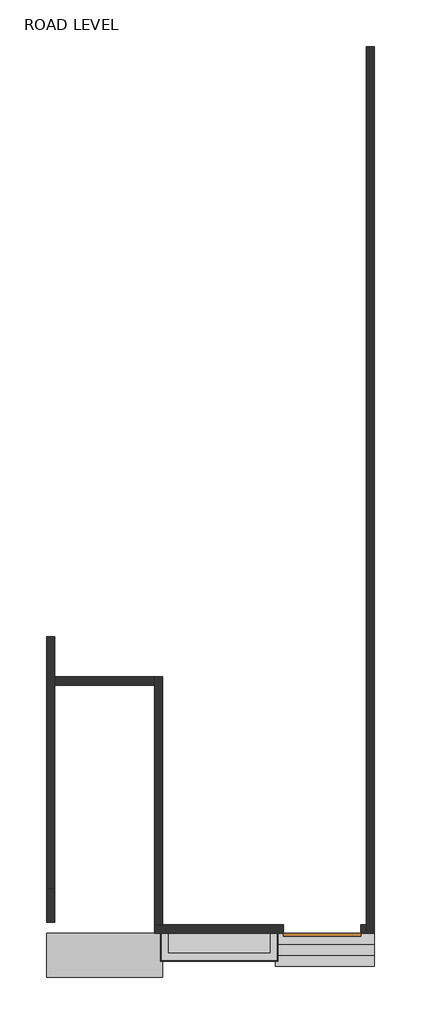
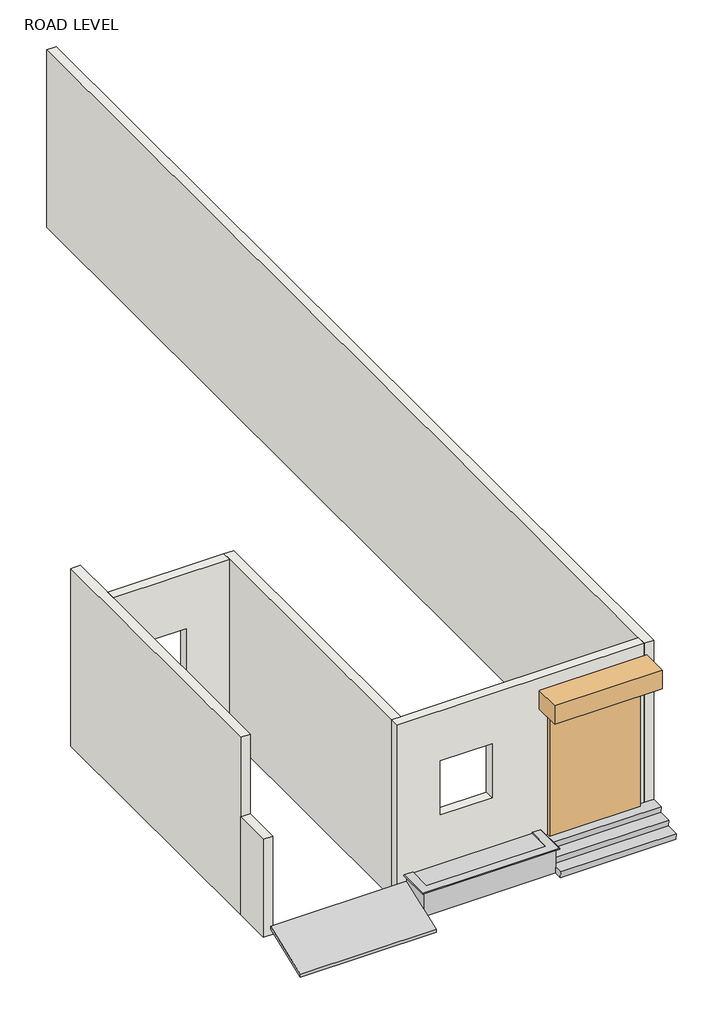
# One storey: 6 walls, 1 door, 1 proxy, 1 ramp, 1 stair flight.
"""IFC4 building model written with IfcOpenShell, lengths in millimetres."""

from ifc_helpers import new_model, si_unit, frame, origin, origin_with_axes, place, context, project, spatial, polyline, outline, extrude, faceted_brep, transform, mapped, element, save
from components import generic_models_2_generic_models_2_8e2cd793, m_door_overhead_rolling_2134_x_3658mm_be0fe279, ramp_3_52017588

model = new_model("IFC4")

# Units and contexts
model_context = context("Model", 3, world=origin())
ifc_project = project(units=[si_unit("LENGTHUNIT", "METRE", prefix="MILLI")], contexts=[model_context])

# Site, building, storey
site = spatial("IfcSite", under=ifc_project)
building = spatial("IfcBuilding", under=site)
storey = spatial("IfcBuildingStorey", under=building, Name="ROAD LEVEL", Elevation=0.0)

# Proxy
placement = place(None, origin())
generic_models_2_generic_models_2_shape = generic_models_2_generic_models_2_8e2cd793(model_context)
element("IfcBuildingElementProxy", 1, Name="Generic Models 2 : Generic Models 2", ObjectType="Generic Models 2 : Generic Models 2", at=placement, inside=storey, context=model_context, shape_type="MappedRepresentation", body=[
    mapped(generic_models_2_generic_models_2_shape, transform((0.0, 0.0, 0.0), x_axis=(1.0, 0.0, 0.0), y_axis=(0.0, 1.0, 0.0), z_axis=(0.0, 0.0, 1.0))),
])

# Door
m_door_overhead_rolling_2134_x_3658mm_shape = m_door_overhead_rolling_2134_x_3658mm_be0fe279(model_context)
element("IfcDoor", 2, ObjectType="M_Door-Overhead-Rolling : 2134 x 3658mm", at=placement, inside=storey, context=model_context, shape_type="MappedRepresentation", body=[
    mapped(m_door_overhead_rolling_2134_x_3658mm_shape, transform((7741.7271331, -11861.4643494, 0.0), x_axis=(1.0, 0.0, 0.0), y_axis=(0.0, 1.0, 0.0), z_axis=(0.0, 0.0, 1.0))),
])

# Ramp
ramp_3_shape = ramp_3_52017588(model_context)
element("IfcRamp", 3, ObjectType="Ramp 3", at=placement, inside=storey, context=model_context, shape_type="MappedRepresentation", body=[
    mapped(ramp_3_shape, transform((0.0, 0.0, 0.0), x_axis=(1.0, 0.0, 0.0), y_axis=(0.0, 1.0, 0.0), z_axis=(0.0, 0.0, 1.0))),
])

# Stair flight
element("IfcStairFlight", 4, ObjectType="3/4\" Nosing", at=placement, inside=storey, context=model_context, shape_type="Brep", body=[
    faceted_brep([(9176.8271331, -12890.1643494, 152.4), (6457.7191987, -12890.1643494, 152.4), (6457.7191987, -12871.1143494, 0.0), (9176.8271331, -12871.1143494, 0.0), (9176.8271331, -12566.3143494, 152.4), (6457.7191987, -12566.3143494, 152.4), (6457.7191987, -12566.3143494, 81.4048417), (6457.7191987, -12729.1240329, 0.0), (9176.8271331, -12729.1240329, 0.0), (9176.8271331, -12566.3143494, 81.4048417), (6457.7191987, -12585.3643494, 304.8), (9176.8271331, -12585.3643494, 304.8), (9176.8271331, -12261.5143494, 304.8), (6457.7191987, -12261.5143494, 304.8), (6457.7191987, -12261.5143494, 233.8048417), (9176.8271331, -12261.5143494, 233.8048417), (6457.7191987, -12280.5643494, 457.2), (9176.8271331, -12280.5643494, 457.2), (9176.8271331, -11975.7643494, 457.2), (6457.7191987, -11975.7643494, 457.2), (6457.7191987, -11975.7643494, 376.6798417), (9176.8271331, -11975.7643494, 376.6798417)], [[[0, 1, 2, 3]], [[1, 0, 4, 5]], [[1, 5, 6, 7, 2]], [[4, 0, 3, 8, 9]], [[10, 11, 12, 13]], [[10, 13, 14, 6, 5]], [[12, 11, 4, 9, 15]], [[5, 4, 11, 10]], [[16, 17, 18, 19]], [[16, 19, 20, 14, 13]], [[18, 17, 12, 15, 21]], [[19, 18, 21, 20]], [[13, 12, 17, 16]], [[3, 2, 7, 8]], [[8, 7, 6, 14, 20, 21, 15, 9]]]),
])

# Walls
element("IfcWall", 5, ObjectType="9\"", at=placement, inside=storey, context=model_context, shape_type="Brep", body=[
    faceted_brep([(8948.2271331, 12408.2356506, 0.0), (8948.2271331, -11747.1643494, 0.0), (8948.2271331, -11975.7643494, 0.0), (8948.2271331, -11975.7643494, 4419.6), (8948.2271331, -11747.1643494, 4419.6), (8948.2271331, 12408.2356506, 4419.6), (9176.8271331, 12408.2356506, 0.0), (9176.8271331, 12408.2356506, 4419.6), (9176.8271331, -11975.7643494, 4419.6), (9176.8271331, -11975.7643494, 0.0)], [[[0, 1, 2, 3, 4, 5]], [[6, 7, 8, 9]], [[2, 1, 0, 6, 9]], [[5, 4, 3, 8, 7]], [[0, 5, 7, 6]], [[3, 2, 9, 8]]]),
])
element("IfcWall", 6, ObjectType="9\"", at=placement, inside=storey, context=model_context, shape_type="Brep", body=[
    faceted_brep([(3118.9271331, -11747.1643494, 4419.6), (3347.5271331, -11747.1643494, 4419.6), (8948.2271331, -11747.1643494, 4419.6), (8948.2271331, -11747.1643494, 0.0), (8808.5271331, -11747.1643494, 0.0), (8808.5271331, -11747.1643494, 3657.6), (6674.9271331, -11747.1643494, 3657.6), (6674.9271331, -11747.1643494, 0.0), (3347.5271331, -11747.1643494, 0.0), (3118.9271331, -11747.1643494, 0.0), (4147.6271331, -11747.1643494, 3175.0), (4147.6271331, -11747.1643494, 1828.8), (5366.8271331, -11747.1643494, 1828.8), (5366.8271331, -11747.1643494, 3175.0), (8948.2271331, -11975.7643494, 4419.6), (3118.9271331, -11975.7643494, 4419.6), (3118.9271331, -11975.7643494, 0.0), (6674.9271331, -11975.7643494, 0.0), (6674.9271331, -11975.7643494, 3657.6), (8808.5271331, -11975.7643494, 3657.6), (8808.5271331, -11975.7643494, 0.0), (8948.2271331, -11975.7643494, 0.0), (4147.6271331, -11975.7643494, 3175.0), (5366.8271331, -11975.7643494, 3175.0), (5366.8271331, -11975.7643494, 1828.8), (4147.6271331, -11975.7643494, 1828.8)], [[[0, 1, 2, 3, 4, 5, 6, 7, 8, 9], [10, 11, 12, 13]], [[14, 15, 16, 17, 18, 19, 20, 21], [22, 23, 24, 25]], [[3, 21, 20, 4]], [[16, 9, 8, 7, 17]], [[2, 1, 0, 15, 14]], [[3, 2, 14, 21]], [[0, 9, 16, 15]], [[19, 5, 4, 20]], [[5, 19, 18, 6]], [[6, 18, 17, 7]], [[11, 10, 22, 25]], [[12, 11, 25, 24]], [[13, 12, 24, 23]], [[10, 13, 23, 22]]]),
])
element("IfcWall", 7, ObjectType="9\"", at=placement, inside=storey, context=model_context, shape_type="Brep", body=[
    faceted_brep([(3347.5271331, -11747.1643494, 0.0), (3347.5271331, -4927.2643494, 0.0), (3347.5271331, -4927.2643494, 4419.6), (3347.5271331, -11747.1643494, 4419.6), (3118.9271331, -11747.1643494, 0.0), (3118.9271331, -11747.1643494, 4419.6), (3118.9271331, -5155.8643494, 4419.6), (3118.9271331, -4927.2643494, 4419.6), (3118.9271331, -4927.2643494, 0.0), (3118.9271331, -5155.8643494, 0.0)], [[[0, 1, 2, 3]], [[4, 5, 6, 7, 8, 9]], [[1, 0, 4, 9, 8]], [[3, 2, 7, 6, 5]], [[0, 3, 5, 4]], [[2, 1, 8, 7]]]),
])
element("IfcWall", 8, ObjectType="9\"", at=placement, inside=storey, context=model_context, shape_type="SweptSolid", body=[
    extrude(outline(polyline([(0.0, 3118.9271331), (4419.6, 3118.9271331), (4419.6, 375.7271331), (0.0, 375.7271331), (0.0, 3118.9271331)]), holes=[polyline([(3048.0, 553.5271331), (3048.0, 2102.9271331), (1828.8, 2102.9271331), (1828.8, 553.5271331), (3048.0, 553.5271331)])]), frame((0.0, -5155.8643494, 0.0), z_axis=(0.0, 1.0, 0.0), x_axis=(0.0, 0.0, 1.0)), (0.0, 0.0, 1.0), 228.6),
])
element("IfcWall", 9, ObjectType="9\"", at=placement, inside=storey, context=model_context, shape_type="Brep", body=[
    faceted_brep([(147.1271331, -3822.3643494, 0.0), (147.1271331, -10756.5643494, 0.0), (147.1271331, -10756.5643494, 2438.4), (147.1271331, -10756.5643494, 4419.6), (147.1271331, -3822.3643494, 4419.6), (375.7271331, -3822.3643494, 0.0), (375.7271331, -3822.3643494, 4419.6), (375.7271331, -4927.2643494, 4419.6), (375.7271331, -5155.8643494, 4419.6), (375.7271331, -10756.5643494, 4419.6), (375.7271331, -10756.5643494, 2438.4), (375.7271331, -10756.5643494, 0.0), (375.7271331, -5155.8643494, 0.0), (375.7271331, -4927.2643494, 0.0)], [[[0, 1, 2, 3, 4]], [[5, 6, 7, 8, 9, 10, 11, 12, 13]], [[1, 0, 5, 13, 12, 11]], [[3, 2, 1, 11, 10, 9]], [[4, 3, 9, 8, 7, 6]], [[0, 4, 6, 5]]]),
])
element("IfcWall", 10, ObjectType="9\"", at=placement, inside=storey, context=model_context, shape_type="SweptSolid", body=[
    extrude(outline(polyline([(147.1271331, -11677.9324242), (147.1271331, -10756.5643494), (375.7271331, -10756.5643494), (375.7271331, -11677.9324242), (147.1271331, -11677.9324242)])), origin_with_axes(), (0.0, 0.0, 1.0), 2438.4),
])

save(model, "model.ifc")

# Revit data of these elements
# Type "M_Door-Overhead-Rolling : 2134 x 3658mm"
#   Type Mark = "8"
#   Construction Type Id = "MDOOR"
#   Assembly Code = "B2030400"
#   Analytic Construction = "Metal"
#   Thickness = 0' - 3.14961"
#   Rough Width [instance default] = 13' - 9.35433"
#   Rough Height [instance default] = 13' - 9.35433"
#   Heat Transfer Coefficient (U) = 0.651978 BTU/(h·ft²·°F)
#   Height [instance default] = 13' - 9.35433"
#   Width [instance default] = 13' - 9.35433"
#   Define Thermal Properties by = 1
#   Function = 1
#   Roller Material = Steel, Paint Finish, Ivory, Matte
#   Roller Box Material = Steel, Paint Finish, Ivory, Matte
#   Visual Light Transmittance = 0
#   Solar Heat Gain Coefficient = 0
#   Wall Closure = (empty or 0)
# Type "Ramp 3"
#   Assembly Code = "B1010600"
#   built-in parameter 1008304 = 0.25 (stored number, unit not read)
#   built-in parameter 1008303 = 30 (stored number, unit not read)
#   built-in parameter 1008301 = 2.66 (stored number, unit not read)
#   Function = 0
#   built-in parameter 1008308 = ramp
# Type "9\""
#   Assembly Code = "B2010"
#   Layers, outside or top first: 0' - 9" no material (function 1)
# Element 1 (IfcBuildingElementProxy, "Generic Models 2 : Generic Models 2")
#   Phase Created = New Construction
#   Materials on its faces: "Roofing, EPDM Membrane", "Oak Flooring", "Tile, Mosaic, Gray"
# Element 2 (IfcDoor, "M_Door-Overhead-Rolling : 2134 x 3658mm")
#   Width = 7' - 0"
#   Rough Width = 7' - 0"
#   Rough Height = 12' - 0"
#   Height = 12' - 0"
#   Phase Created = New Construction
#   Materials on its faces: "Steel, Paint Finish, Ivory, Matte"
# Element 3 (IfcRamp, "Ramp 3")
#   built-in parameter 1007275 = "DN"
#   built-in parameter 1007272 = "UP"
#   Width = 3' - 0"
#   built-in parameter 1007276 = 1
#   built-in parameter 1007274 = 1
#   built-in parameter 1007273 = 1
#   built-in parameter 1007271 = 1
#   Phase Created = New Construction
#   Materials on its faces: "ramp"
# Element 4 (IfcStairFlight, "3/4\" Nosing")
#   Phase Created = New Construction
#   Materials on its faces: "Gypsum Wall Board"
# Elements 5, 6, 7, 8, 9 (IfcWall, "9\"")
#   Top Offset = 0' - 0"
#   Base Offset = 0' - 0"
#   wall height = 14' - 6"
#   Phase Created = New Construction
#   Base Constraint = ROAD LEVEL
#   Top Constraint = FIRST FLOOR LEVEL
#   Materials on its faces: "Default Wall"
# Element 10 (IfcWall, "9\"")
#   Top Offset = 0' - 0"
#   Base Offset = 0' - 0"
#   Unconnected Height = 8' - 0"
#   wall height = 8' - 0"
#   Phase Created = New Construction
#   Base Constraint = ROAD LEVEL
#   Materials on its faces: "Default Wall"
# Materials
#   "Steel, Paint Finish, Ivory, Matte": class "Metal", colour RGB 247 247 239, transparency 0, Description = "Steel, paint finish, ivory, matte", Cost = 0
#   "ramp": class "Generic", colour RGB 123 104 76, transparency 0, Cost = 0
#   "Roofing, EPDM Membrane": class "Generic", colour RGB 127 127 127, transparency 0, Description = "EPDM roof membrane", Cost = 0
#   "Oak Flooring": class "Wood", colour RGB 216 169 114, transparency 0, Description = "Quercus Rubra", Cost = 0
#   "Tile, Mosaic, Gray": class "Generic", colour RGB 127 127 127, transparency 0, Description = "Mosiac tile, gray", Cost = 0
#   "Gypsum Wall Board": class "Generic", colour RGB 228 228 228, transparency 0, Description = "Gypsum Wall Board", Cost = 0
#   "Default Wall": colour RGB 128 128 128, transparency 0, Cost = 0
